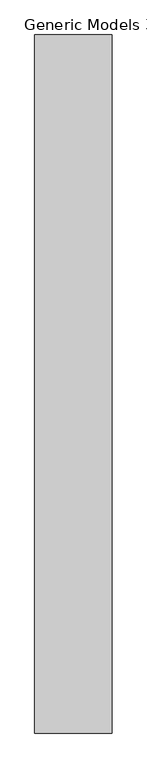
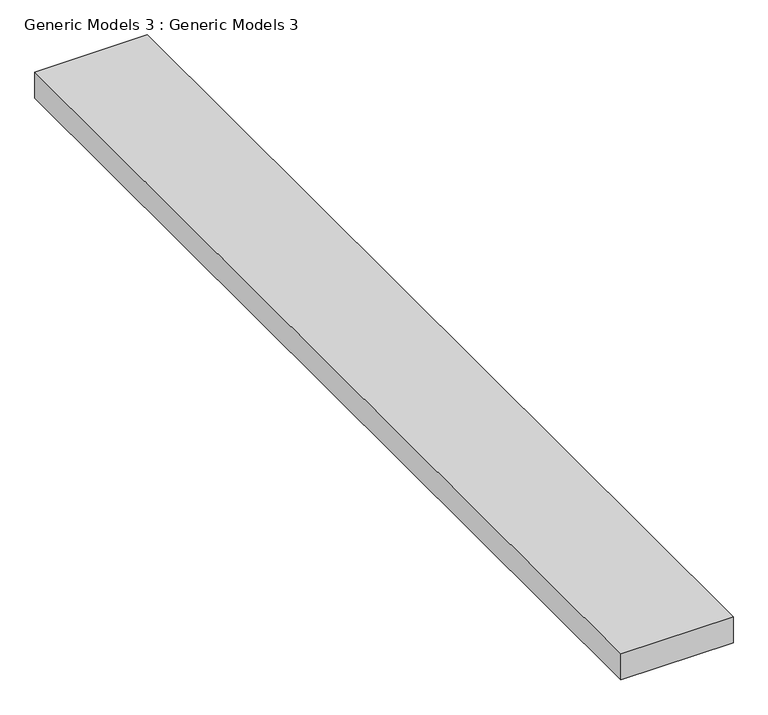
"""IFC4 building model written with IfcOpenShell, lengths in millimetres: proxy geometry, Generic Models 3 : Generic Models 3."""

from ifc_helpers import new_model, si_unit, frame, origin, place, context, project, spatial, polyline, outline, extrude, source, transform, mapped, element, save


def generic_models_3_generic_models_3_6894cc3d(model_context):
    return source(origin(), model_context, "Body", "SweptSolid", [
        extrude(outline(polyline([(-14849.9106439, -7910.6644962), (-14849.9106439, -11912.8112633), (-15292.4161422, -11912.8112633), (-15292.4161422, -7910.6644962), (-14849.9106439, -7910.6644962)])), frame((0.0, 0.0, 5554.8689686), z_axis=(0.0, 0.0, 1.0), x_axis=(1.0, 0.0, 0.0)), (0.0, 0.0, 1.0), 108.596148),
    ])


if __name__ == "__main__":
    model = new_model("IFC4")
    model_context = context("Model", 3, world=origin())
    ifc_project = project(units=[si_unit("LENGTHUNIT", "METRE", prefix="MILLI")], contexts=[model_context])
    site = spatial("IfcSite", under=ifc_project)
    building = spatial("IfcBuilding", under=site)
    placement = place(None, origin())
    generic_models_3_generic_models_3_shape = generic_models_3_generic_models_3_6894cc3d(model_context)
    element("IfcBuildingElementProxy", 1, Name="Generic Models 3 : Generic Models 3", ObjectType="Generic Models 3 : Generic Models 3", at=placement, inside=building, context=model_context, shape_type="MappedRepresentation", body=[
        mapped(generic_models_3_generic_models_3_shape, transform((0.0, 0.0, 0.0), x_axis=(1.0, 0.0, 0.0), y_axis=(0.0, 1.0, 0.0), z_axis=(0.0, 0.0, 1.0))),
    ])
    save(model, "model.ifc")
